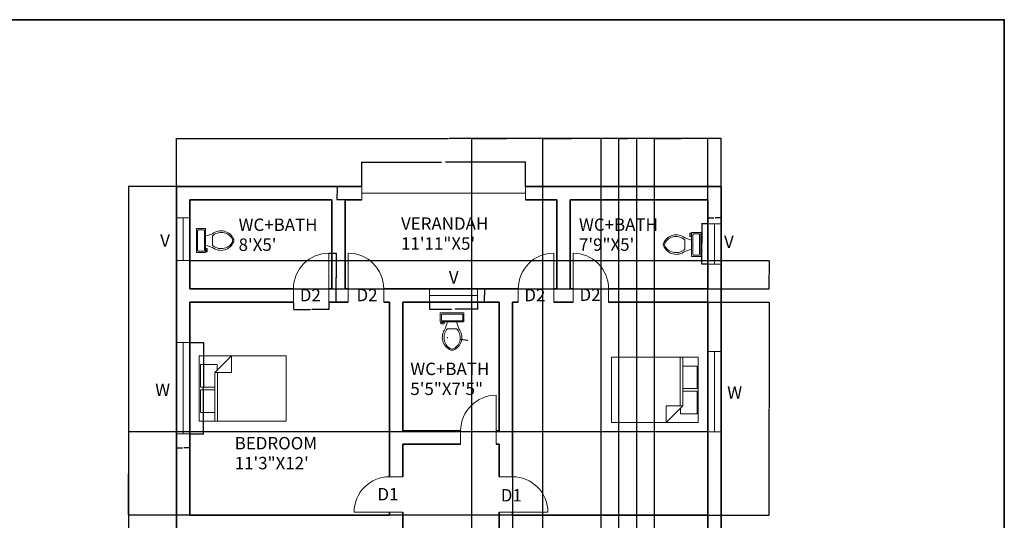
# Model space of a CAD drawing. Units: feet. Extents: x 1654 to 2985, y 1348 to 2230.
# Tile 53 of 53: x 2320 to 2985, y 1892 to 2230. Entities that reach past the tile are written whole.
import ezdxf

# ---------------------------------------------------------------- set-up
doc = ezdxf.new("R2010")
doc.units = ezdxf.units.FT
for name, color, linetype, lineweight in [('A-ANNO-DIMS', 2, 'Continuous', 18), ('A-ANNO-TEXT', 7, 'Continuous', 18), ('A-ANNO-TTLB', 7, 'Continuous', 35), ('A-AREA-IDEN', 7, 'Continuous', 18), ('A-DOOR', 3, 'Continuous', 18), ('A-FLOR-FIXT', 8, 'Continuous', 18), ('A-FURN', 8, 'Continuous', 13), ('A-GLAZ', 4, 'Continuous', 18), ('A-WALL', 7, 'Continuous', 35), ('A-WALL-OPEN', 4, 'Continuous', 18)]:
    doc.layers.add(name, color=color, linetype=linetype, lineweight=lineweight)
doc.styles.get("Standard").update_dxf_attribs({"font": 'arial.ttf'})
doc.dimstyles.get("Standard").update_dxf_attribs({"dimtxt": 0.18, "dimasz": 0.18, "dimexe": 0.18, "dimexo": 0.0625, "dimgap": 0.09, "dimtad": 0, "dimtih": 1, "dimtoh": 1, "dimdec": 4, "dimzin": 0, "dimdsep": 46, "dimtxsty": 'Standard', "dimcen": 0.09, "dimadec": 0, "dimazin": 0, "dimtfac": 1, "dimtdec": 4, "dimtofl": 0, "dimtmove": 0, "dimatfit": 3, "dimfxl": 1, "dimtolj": 1, "dimtzin": 0, "dimarcsym": 0})

# ---------------------------------------------------------------- blocks, each defined once
blk = doc.blocks.new('Toilet - top')
for p, q in [((-10, -8.5), (-8, -8.5)), ((-10, -9.5), (-10, -8.5)), ((-8, -8.5), (-8, -8)), ((-7, -8), (-7, -9.5)), ((-4, -8), (-6, -14)), ((4, -8), (6, -14)), ((9.5, -6), (9.5, -2)), ((-7, -9.5), (-10, -9.5)), ((4, -14), (-4, -14))]:
    blk.add_line(p, q)
blk.add_lwpolyline([(10.5, -8), (10.5, 0), (-10.5, 0), (-10.5, -8)], close=True)
for points in [[(-9.5, -2), (-9.5, -6)], [(8.5, -1), (-8.5, -1)], [(-8.5, -7), (8.5, -7)]]:
    blk.add_lwpolyline(points)
for centre, radius, start, end in [((-8.62, -1.88), 0.884, 81.8699, 188.1301), ((-8.62, -6.12), 0.884, 171.8699, 278.1301), ((8.62, -1.88), 0.884, 351.8699, 98.1301), ((8.62, -6.12), 0.884, 261.8699, 8.1301), ((3.52, -21.58), 12.17, 141.46911, 247.97143), ((4.2, -21.82), 11.33, 136.36773, 238.94682), ((-3.52, -21.58), 12.17, 292.02843, 38.53071), ((-4.2, -21.82), 11.33, 301.05301, 43.63209), ((0, -27.88), 4, 245.73182, 294.26817), ((0, -29), 4, 254.86053, 285.13947)]:
    blk.add_arc(centre, radius, start, end)
blk = doc.blocks.new('Bed - Queen')
for p, q in [((0, -80.00003), (0, 0)), ((0, 0), (59.99999, 0)), ((59.99999, 0), (59.99999, -80.00003)), ((7.99999, -1.2), (28.79998, -1.2)), ((7.99999, -14.4), (7.99999, -1.2)), ((28.79998, -1.2), (28.79998, -14.4)), ((31.19999, -1.2), (51.99999, -1.2)), ((31.19999, -14.4), (31.19999, -1.2)), ((51.99999, -1.2), (51.99999, -16.4)), ((0, -14.4), (44.8, -14.4)), ((44.8, -16.8), (0, -16.8)), ((59.99999, -29.6), (44.8, -14.4)), ((44.8, -14.4), (44.8, -29.6)), ((51.99999, -16.4), (46.79936, -16.4)), ((44.8, -29.6), (59.99999, -29.6)), ((59.99999, -80.00003), (0, -80.00003))]:
    blk.add_line(p, q)
blk = doc.blocks.new('DOOR-D2-SINGLE')
for p, q in [((0, 24), (0, -9)), ((-24, 0), (-24, -9))]:
    blk.add_line(p, q)
blk.add_arc((0, 0), 24, 90, 180)
blk = doc.blocks.new('DOOR-INT-SINGLE')
for p, q in [((0, 24), (9, 24)), ((-24, 0), (9, 0))]:
    blk.add_line(p, q)
blk.add_arc((0, 0), 24, 90, 180)
blk = doc.blocks.new('VENT-BATH-WEST')
for p, q in [((0, 28.76), (9, 28.76)), ((4.5, 28.76), (4.5, 0)), ((0, 0), (9, 0))]:
    blk.add_line(p, q)
blk = doc.blocks.new('OPENING-VERANDAH')
for p, q in [((0, 9), (0, 0)), ((110.69, 9), (110.69, 0)), ((0, 4.5), (110.69, 4.5))]:
    blk.add_line(p, q)
blk = doc.blocks.new('VENT-BATH-EAST')
for p, q in [((0, 27.15), (9, 27.15)), ((4.5, 27.15), (4.5, 0)), ((0, 0), (9, 0))]:
    blk.add_line(p, q)
blk = doc.blocks.new('WIN-BED-WEST')
for p, q in [((0, 61.83), (9, 61.83)), ((4.5, 61.83), (4.5, 0)), ((0, 0), (9, 0))]:
    blk.add_line(p, q)
blk = doc.blocks.new('VENT-BATH-CENTER')
for p, q in [((0, 9), (0, 0)), ((32.4, 9), (32.4, 0)), ((0, 4.5), (32.4, 4.5))]:
    blk.add_line(p, q)
blk = doc.blocks.new('WIN-BED-EAST')
for p, q in [((0, 54.45), (9, 54.45)), ((4.5, 54.45), (4.5, 0)), ((0, 0), (9, 0))]:
    blk.add_line(p, q)
blk = doc.blocks.new('*D28')
at = {"layer": 'A-ANNO-DIMS', "color": 0, "lineweight": -2, "transparency": 16777216}
for p, q in [((2528.77, 2072.25), (2533.84, 2072.25)), ((2533.66, 2072.07), (2533.66, 2055.94)), ((2533.66, 2039.43), (2533.66, 2055.57)), ((2528.77, 2039.25), (2533.84, 2039.25))]:
    blk.add_line(p, q, dxfattribs=at)
at = {"layer": 'A-ANNO-DIMS', "color": 0, "transparency": 16777216}
for points in [[(2533.63, 2072.07), (2533.69, 2072.07), (2533.66, 2072.25)], [(2533.63, 2039.43), (2533.69, 2039.43), (2533.66, 2039.25)]]:
    blk.add_solid(points, dxfattribs=at)
at = {"layer": 'Defpoints', "color": 0, "transparency": 16777216}
for p in [(2528.71, 2072.25), (2533.66, 2072.25), (2528.71, 2039.25)]:
    blk.add_point(p, dxfattribs=at)
at = {"layer": 'A-ANNO-DIMS', "color": 0, "transparency": 16777216, "insert": (2533.66, 2055.75), "char_height": 0.18, "attachment_point": 5}
blk.add_mtext('\\A1;D2 DOOR 33 TYP.', dxfattribs=at)
blk = doc.blocks.new('*D29')
at = {"layer": 'A-ANNO-DIMS', "color": 0, "lineweight": -2, "transparency": 16777216}
for p, q in [((2504.71, 2039.19), (2504.71, 2034.12)), ((2528.71, 2039.19), (2528.71, 2034.12)), ((2504.89, 2034.3), (2516.18, 2034.3)), ((2528.53, 2034.3), (2517.24, 2034.3))]:
    blk.add_line(p, q, dxfattribs=at)
at = {"layer": 'A-ANNO-DIMS', "color": 0, "transparency": 16777216}
for points in [[(2504.89, 2034.33), (2504.89, 2034.27), (2504.71, 2034.3)], [(2528.53, 2034.33), (2528.53, 2034.27), (2528.71, 2034.3)]]:
    blk.add_solid(points, dxfattribs=at)
at = {"layer": 'Defpoints', "color": 0, "transparency": 16777216}
for p in [(2504.71, 2039.25), (2528.71, 2039.25), (2528.71, 2034.3)]:
    blk.add_point(p, dxfattribs=at)
at = {"layer": 'A-ANNO-DIMS', "color": 0, "transparency": 16777216, "insert": (2516.71, 2034.3), "char_height": 0.18, "attachment_point": 5}
blk.add_mtext('\\A1;24 TYP.', dxfattribs=at)
blk = doc.blocks.new('*D50')
at = {"layer": 'A-ANNO-DIMS', "color": 0, "lineweight": -2, "transparency": 16777216}
for p, q in [((2550.87, 2117.32), (2550.87, 2134.04)), ((2551.05, 2133.86), (2604.88, 2133.86)), ((2661.38, 2133.86), (2607.55, 2133.86)), ((2661.56, 2117.32), (2661.56, 2134.04))]:
    blk.add_line(p, q, dxfattribs=at)
at = {"layer": 'A-ANNO-DIMS', "color": 0, "transparency": 16777216}
for points in [[(2551.05, 2133.89), (2551.05, 2133.83), (2550.87, 2133.86)], [(2661.38, 2133.89), (2661.38, 2133.83), (2661.56, 2133.86)]]:
    blk.add_solid(points, dxfattribs=at)
at = {"layer": 'Defpoints', "color": 0, "transparency": 16777216}
for p in [(2550.87, 2133.86), (2550.87, 2117.25), (2661.56, 2117.25)]:
    blk.add_point(p, dxfattribs=at)
at = {"layer": 'A-ANNO-DIMS', "color": 0, "transparency": 16777216, "insert": (2606.21, 2133.86), "char_height": 0.18, "attachment_point": 5}
blk.add_mtext('\\A1;VERANDAH 111 TYP.', dxfattribs=at)
blk = doc.blocks.new('*D51')
at = {"layer": 'A-ANNO-DIMS', "color": 0, "lineweight": -2, "transparency": 16777216}
for p, q in [((2550.81, 2117.25), (2534.08, 2117.25)), ((2534.26, 2117.07), (2534.26, 2112.94)), ((2534.26, 2108.43), (2534.26, 2112.57)), ((2550.81, 2108.25), (2534.08, 2108.25))]:
    blk.add_line(p, q, dxfattribs=at)
at = {"layer": 'A-ANNO-DIMS', "color": 0, "transparency": 16777216}
for points in [[(2534.23, 2117.07), (2534.29, 2117.07), (2534.26, 2117.25)], [(2534.23, 2108.43), (2534.29, 2108.43), (2534.26, 2108.25)]]:
    blk.add_solid(points, dxfattribs=at)
at = {"layer": 'Defpoints', "color": 0, "transparency": 16777216}
for p in [(2550.87, 2117.25), (2534.26, 2108.25), (2550.87, 2108.25)]:
    blk.add_point(p, dxfattribs=at)
at = {"layer": 'A-ANNO-DIMS', "color": 0, "transparency": 16777216, "insert": (2534.26, 2112.75), "char_height": 0.18, "attachment_point": 5}
blk.add_mtext('\\A1;9 TYP.', dxfattribs=at)
blk = doc.blocks.new('*D52')
at = {"layer": 'A-ANNO-DIMS', "color": 0, "lineweight": -2, "transparency": 16777216}
for p, q in [((2784.64, 2092.1), (2780.45, 2092.1)), ((2780.63, 2091.92), (2780.63, 2078.71)), ((2780.63, 2065.13), (2780.63, 2078.34)), ((2784.64, 2064.95), (2780.45, 2064.95))]:
    blk.add_line(p, q, dxfattribs=at)
at = {"layer": 'A-ANNO-DIMS', "color": 0, "transparency": 16777216}
for points in [[(2780.6, 2091.92), (2780.66, 2091.92), (2780.63, 2092.1)], [(2780.6, 2065.13), (2780.66, 2065.13), (2780.63, 2064.95)]]:
    blk.add_solid(points, dxfattribs=at)
at = {"layer": 'Defpoints', "color": 0, "transparency": 16777216}
for p in [(2780.63, 2092.1), (2784.71, 2092.1), (2784.71, 2064.95)]:
    blk.add_point(p, dxfattribs=at)
at = {"layer": 'A-ANNO-DIMS', "color": 0, "transparency": 16777216, "insert": (2780.63, 2078.53), "char_height": 0.18, "attachment_point": 5}
blk.add_mtext('\\A1;EAST VENT 27 TYP.', dxfattribs=at)
blk = doc.blocks.new('*D53')
at = {"layer": 'A-ANNO-DIMS', "color": 0, "lineweight": -2, "transparency": 16777216}
for p, q in [((2784.71, 2092.17), (2784.71, 2096.36)), ((2793.71, 2092.17), (2793.71, 2096.36)), ((2784.89, 2096.18), (2788.75, 2096.18)), ((2793.53, 2096.18), (2789.66, 2096.18))]:
    blk.add_line(p, q, dxfattribs=at)
at = {"layer": 'A-ANNO-DIMS', "color": 0, "transparency": 16777216}
for points in [[(2784.89, 2096.21), (2784.89, 2096.15), (2784.71, 2096.18)], [(2793.53, 2096.21), (2793.53, 2096.15), (2793.71, 2096.18)]]:
    blk.add_solid(points, dxfattribs=at)
at = {"layer": 'Defpoints', "color": 0, "transparency": 16777216}
for p in [(2784.71, 2092.1), (2793.71, 2096.18), (2793.71, 2092.1)]:
    blk.add_point(p, dxfattribs=at)
at = {"layer": 'A-ANNO-DIMS', "color": 0, "transparency": 16777216, "insert": (2789.21, 2096.18), "char_height": 0.18, "attachment_point": 5}
blk.add_mtext('\\A1;9 TYP.', dxfattribs=at)
blk = doc.blocks.new('*D54')
at = {"layer": 'A-ANNO-DIMS', "color": 0, "lineweight": -2, "transparency": 16777216}
for p, q in [((2434.77, 2011.95), (2444.16, 2011.95)), ((2443.98, 2011.77), (2443.98, 1981.22)), ((2443.98, 1950.3), (2443.98, 1980.85)), ((2434.77, 1950.12), (2444.16, 1950.12))]:
    blk.add_line(p, q, dxfattribs=at)
at = {"layer": 'A-ANNO-DIMS', "color": 0, "transparency": 16777216}
for points in [[(2443.95, 2011.77), (2444.01, 2011.77), (2443.98, 2011.95)], [(2443.95, 1950.3), (2444.01, 1950.3), (2443.98, 1950.12)]]:
    blk.add_solid(points, dxfattribs=at)
at = {"layer": 'Defpoints', "color": 0, "transparency": 16777216}
for p in [(2434.71, 2011.95), (2443.98, 2011.95), (2434.71, 1950.12)]:
    blk.add_point(p, dxfattribs=at)
at = {"layer": 'A-ANNO-DIMS', "color": 0, "transparency": 16777216, "insert": (2443.98, 1981.04), "char_height": 0.18, "attachment_point": 5}
blk.add_mtext('\\A1;BEDROOM W 62 TYP.', dxfattribs=at)
blk = doc.blocks.new('*D55')
at = {"layer": 'A-ANNO-DIMS', "color": 0, "lineweight": -2, "transparency": 16777216}
for p, q in [((2425.71, 1950.06), (2425.71, 1940.67)), ((2434.71, 1950.06), (2434.71, 1940.67)), ((2425.89, 1940.85), (2429.75, 1940.85)), ((2434.53, 1940.85), (2430.66, 1940.85))]:
    blk.add_line(p, q, dxfattribs=at)
at = {"layer": 'A-ANNO-DIMS', "color": 0, "transparency": 16777216}
for points in [[(2425.89, 1940.88), (2425.89, 1940.82), (2425.71, 1940.85)], [(2434.53, 1940.88), (2434.53, 1940.82), (2434.71, 1940.85)]]:
    blk.add_solid(points, dxfattribs=at)
at = {"layer": 'Defpoints', "color": 0, "transparency": 16777216}
for p in [(2425.71, 1950.12), (2434.71, 1950.12), (2434.71, 1940.85)]:
    blk.add_point(p, dxfattribs=at)
at = {"layer": 'A-ANNO-DIMS', "color": 0, "transparency": 16777216, "insert": (2430.21, 1940.85), "char_height": 0.18, "attachment_point": 5}
blk.add_mtext('\\A1;9 TYP.', dxfattribs=at)
blk = doc.blocks.new('*D56')
at = {"layer": 'A-ANNO-DIMS', "color": 0, "lineweight": -2, "transparency": 16777216}
for p, q in [((2596.63, 2039.19), (2596.63, 2034.21)), ((2629.03, 2039.19), (2629.03, 2034.21)), ((2596.81, 2034.39), (2611.57, 2034.39)), ((2628.85, 2034.39), (2614.09, 2034.39))]:
    blk.add_line(p, q, dxfattribs=at)
at = {"layer": 'A-ANNO-DIMS', "color": 0, "transparency": 16777216}
for points in [[(2596.81, 2034.42), (2596.81, 2034.36), (2596.63, 2034.39)], [(2628.85, 2034.42), (2628.85, 2034.36), (2629.03, 2034.39)]]:
    blk.add_solid(points, dxfattribs=at)
at = {"layer": 'Defpoints', "color": 0, "transparency": 16777216}
for p in [(2596.63, 2039.25), (2629.03, 2039.25), (2629.03, 2034.39)]:
    blk.add_point(p, dxfattribs=at)
at = {"layer": 'A-ANNO-DIMS', "color": 0, "transparency": 16777216, "insert": (2612.83, 2034.39), "char_height": 0.18, "attachment_point": 5}
blk.add_mtext('\\A1;BATH VENT 32 TYP.', dxfattribs=at)
blk = doc.blocks.new('*D57')
at = {"layer": 'A-ANNO-DIMS', "color": 0, "lineweight": -2, "transparency": 16777216}
for p, q in [((2629.09, 2048.25), (2634.07, 2048.25)), ((2633.89, 2048.07), (2633.89, 2043.94)), ((2633.89, 2039.43), (2633.89, 2043.57)), ((2629.09, 2039.25), (2634.07, 2039.25))]:
    blk.add_line(p, q, dxfattribs=at)
at = {"layer": 'A-ANNO-DIMS', "color": 0, "transparency": 16777216}
for points in [[(2633.86, 2048.07), (2633.92, 2048.07), (2633.89, 2048.25)], [(2633.86, 2039.43), (2633.92, 2039.43), (2633.89, 2039.25)]]:
    blk.add_solid(points, dxfattribs=at)
at = {"layer": 'Defpoints', "color": 0, "transparency": 16777216}
for p in [(2629.03, 2048.25), (2633.89, 2048.25), (2629.03, 2039.25)]:
    blk.add_point(p, dxfattribs=at)
at = {"layer": 'A-ANNO-DIMS', "color": 0, "transparency": 16777216, "insert": (2633.89, 2043.75), "char_height": 0.18, "attachment_point": 5}
blk.add_mtext('\\A1;9 TYP.', dxfattribs=at)
blk = doc.blocks.new('*D78')
at = {"layer": 'A-ANNO-DIMS', "color": 0, "lineweight": -2, "transparency": 16777216}
for p, q in [((2425.71, 2117.32), (2425.71, 2149.88)), ((2425.89, 2149.7), (2609.42, 2149.7)), ((2793.53, 2149.7), (2609.99, 2149.7)), ((2793.71, 2117.32), (2793.71, 2149.88))]:
    blk.add_line(p, q, dxfattribs=at)
at = {"layer": 'A-ANNO-DIMS', "color": 0, "transparency": 16777216}
for points in [[(2425.89, 2149.73), (2425.89, 2149.67), (2425.71, 2149.7)], [(2793.53, 2149.73), (2793.53, 2149.67), (2793.71, 2149.7)]]:
    blk.add_solid(points, dxfattribs=at)
at = {"layer": 'Defpoints', "color": 0, "transparency": 16777216}
for p in [(2793.71, 2149.7), (2425.71, 2117.25), (2793.71, 2117.25)]:
    blk.add_point(p, dxfattribs=at)
at = {"layer": 'A-ANNO-DIMS', "color": 0, "transparency": 16777216, "insert": (2609.71, 2149.7), "char_height": 0.18, "attachment_point": 5}
blk.add_mtext('\\A1;368', dxfattribs=at)
blk = doc.blocks.new('*D79')
at = {"layer": 'A-ANNO-DIMS', "color": 0, "lineweight": -2, "transparency": 16777216}
for p, q in [((2425.64, 2117.25), (2393.08, 2117.25)), ((2393.26, 2117.07), (2393.26, 1820.44)), ((2393.26, 1523.43), (2393.26, 1820.07)), ((2425.64, 1523.25), (2393.08, 1523.25))]:
    blk.add_line(p, q, dxfattribs=at)
at = {"layer": 'A-ANNO-DIMS', "color": 0, "transparency": 16777216}
for points in [[(2393.23, 2117.07), (2393.29, 2117.07), (2393.26, 2117.25)], [(2393.23, 1523.43), (2393.29, 1523.43), (2393.26, 1523.25)]]:
    blk.add_solid(points, dxfattribs=at)
at = {"layer": 'Defpoints', "color": 0, "transparency": 16777216}
for p in [(2393.26, 2117.25), (2425.71, 2117.25), (2425.71, 1523.25)]:
    blk.add_point(p, dxfattribs=at)
at = {"layer": 'A-ANNO-DIMS', "color": 0, "transparency": 16777216, "insert": (2393.26, 1820.25), "char_height": 0.18, "attachment_point": 5}
blk.add_mtext('\\A1;594', dxfattribs=at)
blk = doc.blocks.new('*D82')
at = {"layer": 'A-ANNO-DIMS', "color": 0, "lineweight": -2, "transparency": 16777216}
for p, q in [((2652.71, 2039.19), (2652.71, 1490.62)), ((2784.71, 2039.19), (2784.71, 1490.62)), ((2652.89, 1490.8), (2718.43, 1490.8)), ((2784.53, 1490.8), (2718.99, 1490.8))]:
    blk.add_line(p, q, dxfattribs=at)
at = {"layer": 'A-ANNO-DIMS', "color": 0, "transparency": 16777216}
for points in [[(2652.89, 1490.83), (2652.89, 1490.77), (2652.71, 1490.8)], [(2784.53, 1490.83), (2784.53, 1490.77), (2784.71, 1490.8)]]:
    blk.add_solid(points, dxfattribs=at)
at = {"layer": 'Defpoints', "color": 0, "transparency": 16777216}
for p in [(2652.71, 2039.25), (2784.71, 2039.25), (2784.71, 1490.8)]:
    blk.add_point(p, dxfattribs=at)
at = {"layer": 'A-ANNO-DIMS', "color": 0, "transparency": 16777216, "insert": (2718.71, 1490.8), "char_height": 0.18, "attachment_point": 5}
blk.add_mtext('\\A1;132', dxfattribs=at)
blk = doc.blocks.new('*D83')
at = {"layer": 'A-ANNO-DIMS', "color": 0, "lineweight": -2, "transparency": 16777216}
for p, q in [((2784.77, 2039.25), (2826.34, 2039.25)), ((2826.16, 2039.07), (2826.16, 1967.44)), ((2826.16, 1895.43), (2826.16, 1967.07)), ((2784.77, 1895.25), (2826.34, 1895.25))]:
    blk.add_line(p, q, dxfattribs=at)
at = {"layer": 'A-ANNO-DIMS', "color": 0, "transparency": 16777216}
for points in [[(2826.13, 2039.07), (2826.19, 2039.07), (2826.16, 2039.25)], [(2826.13, 1895.43), (2826.19, 1895.43), (2826.16, 1895.25)]]:
    blk.add_solid(points, dxfattribs=at)
at = {"layer": 'Defpoints', "color": 0, "transparency": 16777216}
for p in [(2784.71, 2039.25), (2826.16, 2039.25), (2784.71, 1895.25)]:
    blk.add_point(p, dxfattribs=at)
at = {"layer": 'A-ANNO-DIMS', "color": 0, "transparency": 16777216, "insert": (2826.16, 1967.25), "char_height": 0.18, "attachment_point": 5}
blk.add_mtext('\\A1;144', dxfattribs=at)
blk = doc.blocks.new('*D84')
at = {"layer": 'A-ANNO-DIMS', "color": 0, "lineweight": -2, "transparency": 16777216}
for p, q in [((2625.24, 1565.32), (2625.24, 2149.88)), ((2625.42, 2149.7), (2649.01, 2149.7)), ((2673.06, 2149.7), (2649.46, 2149.7)), ((2673.24, 1565.32), (2673.24, 2149.88))]:
    blk.add_line(p, q, dxfattribs=at)
at = {"layer": 'A-ANNO-DIMS', "color": 0, "transparency": 16777216}
for points in [[(2625.42, 2149.73), (2625.42, 2149.67), (2625.24, 2149.7)], [(2673.06, 2149.73), (2673.06, 2149.67), (2673.24, 2149.7)]]:
    blk.add_solid(points, dxfattribs=at)
at = {"layer": 'Defpoints', "color": 0, "transparency": 16777216}
for p in [(2673.24, 2149.7), (2625.24, 1565.25), (2673.24, 1565.25)]:
    blk.add_point(p, dxfattribs=at)
at = {"layer": 'A-ANNO-DIMS', "color": 0, "transparency": 16777216, "insert": (2649.24, 2149.7), "char_height": 0.18, "attachment_point": 5}
blk.add_mtext('\\A1;48', dxfattribs=at)
blk = doc.blocks.new('*D85')
at = {"layer": 'A-ANNO-DIMS', "color": 0, "lineweight": -2, "transparency": 16777216}
for p, q in [((2673.24, 1565.32), (2673.24, 2149.88)), ((2673.42, 2149.7), (2692.58, 2149.7)), ((2712.53, 2149.7), (2693.36, 2149.7)), ((2712.71, 1565.32), (2712.71, 2149.88))]:
    blk.add_line(p, q, dxfattribs=at)
at = {"layer": 'A-ANNO-DIMS', "color": 0, "transparency": 16777216}
for points in [[(2673.42, 2149.73), (2673.42, 2149.67), (2673.24, 2149.7)], [(2712.53, 2149.73), (2712.53, 2149.67), (2712.71, 2149.7)]]:
    blk.add_solid(points, dxfattribs=at)
at = {"layer": 'Defpoints', "color": 0, "transparency": 16777216}
for p in [(2712.71, 2149.7), (2673.24, 1565.25), (2712.71, 1565.25)]:
    blk.add_point(p, dxfattribs=at)
at = {"layer": 'A-ANNO-DIMS', "color": 0, "transparency": 16777216, "insert": (2692.97, 2149.7), "char_height": 0.18, "attachment_point": 5}
blk.add_mtext('\\A1;39.47', dxfattribs=at)
blk = doc.blocks.new('*D86')
at = {"layer": 'A-ANNO-DIMS', "color": 0, "lineweight": -2, "transparency": 16777216}
for p, q in [((2748.71, 1616.32), (2748.71, 2149.88)), ((2748.89, 2149.7), (2766.49, 2149.7)), ((2784.53, 2149.7), (2766.92, 2149.7)), ((2784.71, 1607.32), (2784.71, 2149.88))]:
    blk.add_line(p, q, dxfattribs=at)
at = {"layer": 'A-ANNO-DIMS', "color": 0, "transparency": 16777216}
for points in [[(2748.89, 2149.73), (2748.89, 2149.67), (2748.71, 2149.7)], [(2784.53, 2149.73), (2784.53, 2149.67), (2784.71, 2149.7)]]:
    blk.add_solid(points, dxfattribs=at)
at = {"layer": 'Defpoints', "color": 0, "transparency": 16777216}
for p in [(2784.71, 2149.7), (2748.71, 1616.25), (2784.71, 1607.25)]:
    blk.add_point(p, dxfattribs=at)
at = {"layer": 'A-ANNO-DIMS', "color": 0, "transparency": 16777216, "insert": (2766.71, 2149.7), "char_height": 0.18, "attachment_point": 5}
blk.add_mtext('\\A1;36', dxfattribs=at)
blk = doc.blocks.new('*D87')
at = {"layer": 'A-ANNO-DIMS', "color": 0, "lineweight": -2, "transparency": 16777216}
for p, q in [((2724.71, 1565.32), (2724.71, 2149.88)), ((2724.89, 2149.7), (2730.5, 2149.7)), ((2736.53, 2149.7), (2730.92, 2149.7)), ((2736.71, 1565.32), (2736.71, 2149.88))]:
    blk.add_line(p, q, dxfattribs=at)
at = {"layer": 'A-ANNO-DIMS', "color": 0, "transparency": 16777216}
for points in [[(2724.89, 2149.73), (2724.89, 2149.67), (2724.71, 2149.7)], [(2736.53, 2149.73), (2736.53, 2149.67), (2736.71, 2149.7)]]:
    blk.add_solid(points, dxfattribs=at)
at = {"layer": 'Defpoints', "color": 0, "transparency": 16777216}
for p in [(2736.71, 2149.7), (2724.71, 1565.25), (2736.71, 1565.25)]:
    blk.add_point(p, dxfattribs=at)
at = {"layer": 'A-ANNO-DIMS', "color": 0, "transparency": 16777216, "insert": (2730.71, 2149.7), "char_height": 0.18, "attachment_point": 5}
blk.add_mtext('\\A1;12', dxfattribs=at)
blk = doc.blocks.new('*D93')
at = {"layer": 'A-ANNO-DIMS', "color": 0, "lineweight": -2, "transparency": 16777216}
for p, q in [((2434.77, 2067.34), (2826.34, 2067.34)), ((2826.16, 2067.16), (2826.16, 2057.98)), ((2826.16, 2048.43), (2826.16, 2057.62)), ((2434.77, 2048.25), (2826.34, 2048.25))]:
    blk.add_line(p, q, dxfattribs=at)
at = {"layer": 'A-ANNO-DIMS', "color": 0, "transparency": 16777216}
for points in [[(2826.13, 2067.16), (2826.19, 2067.16), (2826.16, 2067.34)], [(2826.13, 2048.43), (2826.19, 2048.43), (2826.16, 2048.25)]]:
    blk.add_solid(points, dxfattribs=at)
at = {"layer": 'Defpoints', "color": 0, "transparency": 16777216}
for p in [(2434.71, 2067.34), (2826.16, 2067.34), (2434.71, 2048.25)]:
    blk.add_point(p, dxfattribs=at)
at = {"layer": 'A-ANNO-DIMS', "color": 0, "transparency": 16777216, "insert": (2826.16, 2057.8), "char_height": 0.18, "attachment_point": 5}
blk.add_mtext('\\A1;19.084', dxfattribs=at)
blk = doc.blocks.new('*D95')
at = {"layer": 'A-ANNO-DIMS', "color": 0, "lineweight": -2, "transparency": 16777216}
for p, q in [((2784.64, 1951.49), (2393.08, 1951.49)), ((2393.26, 1951.31), (2393.26, 1923.55)), ((2393.26, 1895.43), (2393.26, 1923.19)), ((2784.64, 1895.25), (2393.08, 1895.25))]:
    blk.add_line(p, q, dxfattribs=at)
at = {"layer": 'A-ANNO-DIMS', "color": 0, "transparency": 16777216}
for points in [[(2393.23, 1951.31), (2393.29, 1951.31), (2393.26, 1951.49)], [(2393.23, 1895.43), (2393.29, 1895.43), (2393.26, 1895.25)]]:
    blk.add_solid(points, dxfattribs=at)
at = {"layer": 'Defpoints', "color": 0, "transparency": 16777216}
for p in [(2393.26, 1951.49), (2784.71, 1951.49), (2784.71, 1895.25)]:
    blk.add_point(p, dxfattribs=at)
at = {"layer": 'A-ANNO-DIMS', "color": 0, "transparency": 16777216, "insert": (2393.26, 1923.37), "char_height": 0.18, "attachment_point": 5}
blk.add_mtext('\\A1;56.23', dxfattribs=at)
blk = doc.blocks.new('*D113')
at = {"layer": 'A-ANNO-DIMS', "color": 0, "lineweight": -2, "transparency": 16777216}
for p, q in [((2608.65, 2015.2), (2608.83, 2015.2)), ((2608.74, 2015.11), (2608.74, 2015.29)), ((2622.48, 2013.35), (2617.51, 2014.02))]:
    blk.add_line(p, q, dxfattribs=at)
at = {"layer": 'A-ANNO-DIMS', "color": 0, "transparency": 16777216}
blk.add_solid([(2617.51, 2014.05), (2617.5, 2013.99), (2617.33, 2014.04)], dxfattribs=at)
at = {"layer": 'Defpoints', "color": 0, "transparency": 16777216}
for p in [(2608.74, 2015.2), (2617.33, 2014.04)]:
    blk.add_point(p, dxfattribs=at)
at = {"layer": 'A-ANNO-DIMS', "color": 0, "transparency": 16777216, "insert": (2623.22, 2013.35), "char_height": 0.18, "attachment_point": 5}
blk.add_mtext('\\A1;12X R8.669', dxfattribs=at)

msp = doc.modelspace()

# ---------------------------------------------------------------- linework, layer by layer
at = {"layer": 'A-ANNO-TTLB'}
msp.add_lwpolyline([(1654.1997, 2230.0267), (2985.175, 2230.0267), (2985.175, 1348.1324), (1654.1997, 1348.1324)], close=True, dxfattribs=at)
at = {"layer": 'A-WALL'}
for p, q in [((2425.7058, 2117.2549), (2550.8676, 2117.2549)), ((2425.7058, 2048.2549), (2425.7058, 2117.2549)), ((2425.7058, 2117.2549), (2425.7058, 1565.2549)), ((2539.7058, 2117.2549), (2550.8676, 2117.2549)), ((2661.5555, 2117.2549), (2793.7058, 2117.2549)), ((2661.5555, 2117.2549), (2682.7058, 2117.2549)), ((2691.7058, 2117.2549), (2793.7058, 2117.2549)), ((2793.7058, 2117.2549), (2793.7058, 1742.2549)), ((2434.7058, 2108.2549), (2530.7058, 2108.2549)), ((2434.7058, 2048.2549), (2434.7058, 2108.2549)), ((2530.7058, 2108.2549), (2530.7058, 2048.2549)), ((2539.7058, 2108.2549), (2539.7058, 2048.2549)), ((2539.7058, 2108.2549), (2550.8676, 2108.2549)), ((2661.5555, 2108.2549), (2682.7058, 2108.2549)), ((2682.7058, 2108.2549), (2682.7058, 2048.2549)), ((2691.7058, 2108.2549), (2691.7058, 2048.2549)), ((2691.7058, 2108.2549), (2784.7058, 2108.2549)), ((2784.7058, 2108.2549), (2784.7058, 2048.2549)), ((2504.7058, 2048.2549), (2434.7058, 2048.2549)), ((2530.7058, 2048.2549), (2528.7058, 2048.2549)), ((2541.7058, 2048.2549), (2539.7058, 2048.2549)), ((2656.7058, 2048.2549), (2565.7058, 2048.2549)), ((2682.7058, 2048.2549), (2680.7058, 2048.2549)), ((2693.7058, 2048.2549), (2691.7058, 2048.2549)), ((2784.7058, 2048.2549), (2717.7058, 2048.2549)), ((2504.7058, 2039.2549), (2434.7058, 2039.2549)), ((2434.7058, 2039.2549), (2434.7058, 1895.2549)), ((2541.7058, 2039.2549), (2528.7058, 2039.2549)), ((2541.7058, 2039.2549), (2539.7058, 2039.2549)), ((2569.7058, 2039.2549), (2565.7058, 2039.2549)), ((2569.7058, 2039.2549), (2565.7058, 2039.2549)), ((2569.7058, 1921.2549), (2569.7058, 2039.2549)), ((2643.7058, 2039.2549), (2578.7058, 2039.2549)), ((2578.7058, 1952.2549), (2578.7058, 2039.2549)), ((2643.7058, 1952.2549), (2643.7058, 2039.2549)), ((2656.7058, 2039.2549), (2652.7058, 2039.2549)), ((2652.7058, 1921.2549), (2652.7058, 2039.2549)), ((2693.7058, 2039.2549), (2680.7058, 2039.2549)), ((2693.7058, 2039.2549), (2691.7058, 2039.2549)), ((2784.7058, 2039.2549), (2717.7058, 2039.2549)), ((2784.7058, 2039.2549), (2717.7058, 2039.2549)), ((2784.7058, 2039.2549), (2784.7058, 1895.2549)), ((2793.7058, 2039.2549), (2793.7058, 1895.2549)), ((2617.7058, 1952.2549), (2578.7058, 1952.2549)), ((2643.7058, 1952.2549), (2641.7058, 1952.2549)), ((2617.7058, 1943.2549), (2578.7058, 1943.2549)), ((2578.7058, 1921.2549), (2578.7058, 1943.2549)), ((2643.7058, 1943.2549), (2641.7058, 1943.2549)), ((2643.7058, 1921.2549), (2643.7058, 1943.2549)), ((2569.7058, 1895.2549), (2569.7058, 1897.2549)), ((2578.7058, 1886.2549), (2578.7058, 1897.2549)), ((2643.7058, 1895.2549), (2643.7058, 1897.2549)), ((2652.7058, 1895.2549), (2652.7058, 1897.2549)), ((2434.7058, 1895.2549), (2569.7058, 1895.2549)), ((2643.7058, 1895.2549), (2643.7058, 1886.2549)), ((2784.7058, 1895.2549), (2652.7058, 1895.2549))]:
    msp.add_line(p, q, dxfattribs=at)

# ---------------------------------------------------------------- block references
at = {"layer": 'A-DOOR'}
for name, p in [('DOOR-D2-SINGLE', (2528.7058, 2048.2549)), ('DOOR-D2-SINGLE', (2680.7058, 2048.2549)), ('DOOR-INT-SINGLE', (2569.7058, 1897.2549))]:
    msp.add_blockref(name, p, dxfattribs=at)
at = {"layer": 'A-DOOR', "extrusion": (0, 0, -1), "zscale": -1}
for name, p in [('DOOR-D2-SINGLE', (-2541.7058, 2048.2549)), ('DOOR-D2-SINGLE', (-2693.7058, 2048.2549)), ('DOOR-INT-SINGLE', (-2652.7058, 1897.2549))]:
    msp.add_blockref(name, p, dxfattribs=at)
at = {"layer": 'A-DOOR', "extrusion": (0, 0, -1), "zscale": -1, "rotation": 270.0000000000017}
msp.add_blockref('DOOR-INT-SINGLE', (-2641.7058, 1952.2549), dxfattribs=at)
at = {"layer": 'A-FLOR-FIXT', "xscale": 0.7651522138144634, "yscale": 0.7651522138144634, "zscale": 0.7651522138144634}
for p, rotation in [((2439.1813, 2080.7996), 90), ((2779.9575, 2078.0929), 270)]:
    msp.add_blockref('Toilet - top', p, dxfattribs=dict(at, rotation=rotation))
msp.add_blockref('Toilet - top', (2611.9504, 2031.8905), dxfattribs=at)
at = {"layer": 'A-FURN', "xscale": 0.7339343441631778, "yscale": 0.7339343441631778, "zscale": 0.7339343441631778}
for p, rotation in [((2441.0628, 1958.8411), 90), ((2778.3599, 2001.9019), 270)]:
    msp.add_blockref('Bed - Queen', p, dxfattribs=dict(at, rotation=rotation))
at = {"layer": 'A-GLAZ'}
for name, p in [('VENT-BATH-WEST', (2425.7054, 2067.339)), ('VENT-BATH-EAST', (2784.7054, 2064.949)), ('VENT-BATH-CENTER', (2596.6294, 2039.255)), ('WIN-BED-WEST', (2425.7054, 1950.122)), ('WIN-BED-EAST', (2784.7054, 1951.488))]:
    msp.add_blockref(name, p, dxfattribs=at)
at = {"layer": 'A-WALL-OPEN', "rotation": 180}
msp.add_blockref('OPENING-VERANDAH', (2661.5557, 2117.2549), dxfattribs=at)

# ---------------------------------------------------------------- texts
at = {"layer": 'A-ANNO-TEXT'}
for s, height, p in [('V', 8.3811, (2414.6389, 2076.6892)), ('V', 8.3811, (2795.7438, 2075.7989)), ('V', 8.3811, (2609.7577, 2051.7341)), ('D2', 8.38114, (2509.0145, 2039.7278)), ('D2', 8.38114, (2547.3527, 2039.8017)), ('D2', 8.38114, (2660.783, 2039.7473)), ('D2', 8.38114, (2698.0826, 2039.9826)), ('W', 8.3811, (2411.288, 1975.7867)), ('W', 8.3811, (2797.8989, 1973.858)), ('D1', 8.38114, (2561.4803, 1905.2296)), ('D1', 8.38114, (2644.874, 1904.4938))]:
    msp.add_text(s, height=height, dxfattribs=at).set_placement(p)
at = {"layer": 'A-AREA-IDEN'}
for s, p in [('VERANDAH', (2577.4476, 2088.049)), ('WC+BATH', (2467.6532, 2087.2734)), ('WC+BATH', (2697.7117, 2087.3504)), ('11\'11"X5\'', (2577.4476, 2074.5854)), ("8'X5'", (2467.6532, 2073.8098)), ('7\'9"X5\'', (2697.7117, 2073.8868)), ('WC+BATH', (2583.7182, 1989.9081)), ('5\'5"X7\'5"', (2583.7182, 1976.4445)), ('BEDROOM', (2465.0141, 1939.6855)), ('11\'3"X12\'', (2465.0141, 1926.222))]:
    msp.add_text(s, height=8.38114, dxfattribs=at).set_placement(p)

# ---------------------------------------------------------------- dimensions: what is measured, and where the dimension line sits
at = {"layer": 'A-ANNO-DIMS'}
for base, p1, p2, override, picture, middle in [((2793.7058, 2149.7049), (2425.7058, 2117.2549), (2793.7058, 2117.2549), {"dimdec": 0, "dimlfac": 1, "dimrnd": 0, "dimzin": 0, "dimdsep": 46, "dimlunit": 2}, '*D78', (2609.7058, 2149.7049)), ((2673.2353, 2149.7049), (2625.2353, 1565.2549), (2673.2353, 1565.2549), {"dimdec": 0, "dimlfac": 1, "dimrnd": 0, "dimzin": 0, "dimdsep": 46, "dimlunit": 2}, '*D84', (2649.2353, 2149.7049)), ((2712.7058, 2149.7049), (2673.2353, 1565.2549), (2712.7058, 1565.2549), {"dimdec": 2, "dimlfac": 1, "dimrnd": 0, "dimzin": 0, "dimdsep": 46, "dimlunit": 2}, '*D85', (2692.9706, 2149.7049)), ((2736.7058, 2149.7049), (2724.7058, 1565.2549), (2736.7058, 1565.2549), {"dimdec": 0, "dimlfac": 1, "dimrnd": 0, "dimzin": 0, "dimdsep": 46, "dimlunit": 2}, '*D87', (2730.7058, 2149.7049)), ((2784.7058, 2149.7049), (2748.7058, 1616.2549), (2784.7058, 1607.2549), {"dimdec": 0, "dimlfac": 1, "dimrnd": 0, "dimzin": 0, "dimdsep": 46, "dimlunit": 2}, '*D86', (2766.7058, 2149.7049)), ((2784.7058, 1490.8049), (2652.7058, 2039.2549), (2784.7058, 2039.2549), {"dimdec": 0, "dimlfac": 1, "dimrnd": 0, "dimzin": 0, "dimdsep": 46, "dimlunit": 2}, '*D82', (2718.7058, 1490.8049))]:
    dim = msp.add_linear_dim(base=base, p1=p1, p2=p2, dimstyle='Standard', override=override, dxfattribs=at)
    dim.commit()
    dim.dimension.update_dxf_attribs({"geometry": picture, "text_midpoint": middle})
for base, p1, p2, angle, text, picture, middle in [((2550.8676, 2133.8581), (2661.5555, 2117.2549), (2550.8676, 2117.2549), 180, 'VERANDAH <> TYP.', '*D50', (2606.2116, 2133.8581)), ((2534.2645, 2108.2549), (2550.8676, 2117.2549), (2550.8676, 2108.2549), 270, '<> TYP.', '*D51', (2534.2645, 2112.7549)), ((2780.6327, 2092.1027), (2784.7058, 2064.9486), (2784.7058, 2092.1027), 90, 'EAST VENT <> TYP.', '*D52', (2780.6327, 2078.5257)), ((2533.6558, 2072.2549), (2528.7058, 2039.2549), (2528.7058, 2072.2549), 90, 'D2 DOOR <> TYP.', '*D28', (2533.6558, 2055.7549)), ((2633.8905, 2048.2549), (2629.0304, 2039.2549), (2629.0304, 2048.2549), 90, '<> TYP.', '*D57', (2633.8905, 2043.7549)), ((2443.9803, 2011.9524), (2434.7058, 1950.1224), (2434.7058, 2011.9524), 90, 'BEDROOM W <> TYP.', '*D54', (2443.9803, 1981.0374))]:
    dim = msp.add_linear_dim(base=base, p1=p1, p2=p2, angle=angle, text=text, dimstyle='Standard', override={"dimdec": 0, "dimlfac": 1, "dimrnd": 0, "dimzin": 0, "dimdsep": 46, "dimlunit": 2}, dxfattribs=at)
    dim.commit()
    dim.dimension.update_dxf_attribs({"geometry": picture, "text_midpoint": middle})
for base, p1, p2, override, picture, middle in [((2393.2558, 2117.2549), (2425.7058, 1523.2549), (2425.7058, 2117.2549), {"dimdec": 0, "dimlfac": 1, "dimrnd": 0, "dimzin": 0, "dimdsep": 46, "dimlunit": 2}, '*D79', (2393.2558, 1820.2549)), ((2826.1558, 2067.3393), (2434.7058, 2048.2549), (2434.7058, 2067.3393), {"dimdec": 3, "dimlfac": 1, "dimrnd": 0, "dimzin": 0, "dimdsep": 46, "dimlunit": 2}, '*D93', (2826.1558, 2057.7971)), ((2826.1558, 2039.2549), (2784.7058, 1895.2549), (2784.7058, 2039.2549), {"dimdec": 0, "dimlfac": 1, "dimrnd": 0, "dimzin": 0, "dimdsep": 46, "dimlunit": 2}, '*D83', (2826.1558, 1967.2549)), ((2393.2558, 1951.4875), (2784.7058, 1895.2549), (2784.7058, 1951.4875), {"dimdec": 2, "dimlfac": 1, "dimrnd": 0, "dimzin": 0, "dimdsep": 46, "dimlunit": 2}, '*D95', (2393.2558, 1923.3712))]:
    dim = msp.add_linear_dim(base=base, p1=p1, p2=p2, angle=90, dimstyle='Standard', override=override, dxfattribs=at)
    dim.commit()
    dim.dimension.update_dxf_attribs({"geometry": picture, "text_midpoint": middle})
for base, p1, p2, text, picture, middle in [((2793.7058, 2096.1758), (2784.7058, 2092.1027), (2793.7058, 2092.1027), '<> TYP.', '*D53', (2789.2058, 2096.1758)), ((2528.7058, 2034.3049), (2504.7058, 2039.2549), (2528.7058, 2039.2549), '<> TYP.', '*D29', (2516.7058, 2034.3049)), ((2629.0304, 2034.3948), (2596.6294, 2039.2549), (2629.0304, 2039.2549), 'BATH VENT <> TYP.', '*D56', (2612.8299, 2034.3948)), ((2434.7058, 1940.8479), (2425.7058, 1950.1224), (2434.7058, 1950.1224), '<> TYP.', '*D55', (2430.2058, 1940.8479))]:
    dim = msp.add_linear_dim(base=base, p1=p1, p2=p2, text=text, dimstyle='Standard', override={"dimdec": 0, "dimlfac": 1, "dimrnd": 0, "dimzin": 0, "dimdsep": 46, "dimlunit": 2}, dxfattribs=at)
    dim.commit()
    dim.dimension.update_dxf_attribs({"geometry": picture, "text_midpoint": middle})
dim = msp.add_radius_dim(center=(2608.7368, 2015.1969), mpoint=(2617.3281, 2014.042), text='12X <>', dimstyle='Standard', override={"dimdec": 3, "dimlfac": 1, "dimrnd": 0, "dimzin": 0, "dimdsep": 46, "dimlunit": 2}, dxfattribs=at)
dim.commit()
dim.dimension.update_dxf_attribs({"geometry": '*D113', "text_midpoint": (2622.4829, 2013.349), "dimtype": 164})

doc.saveas('drawing.dxf')
